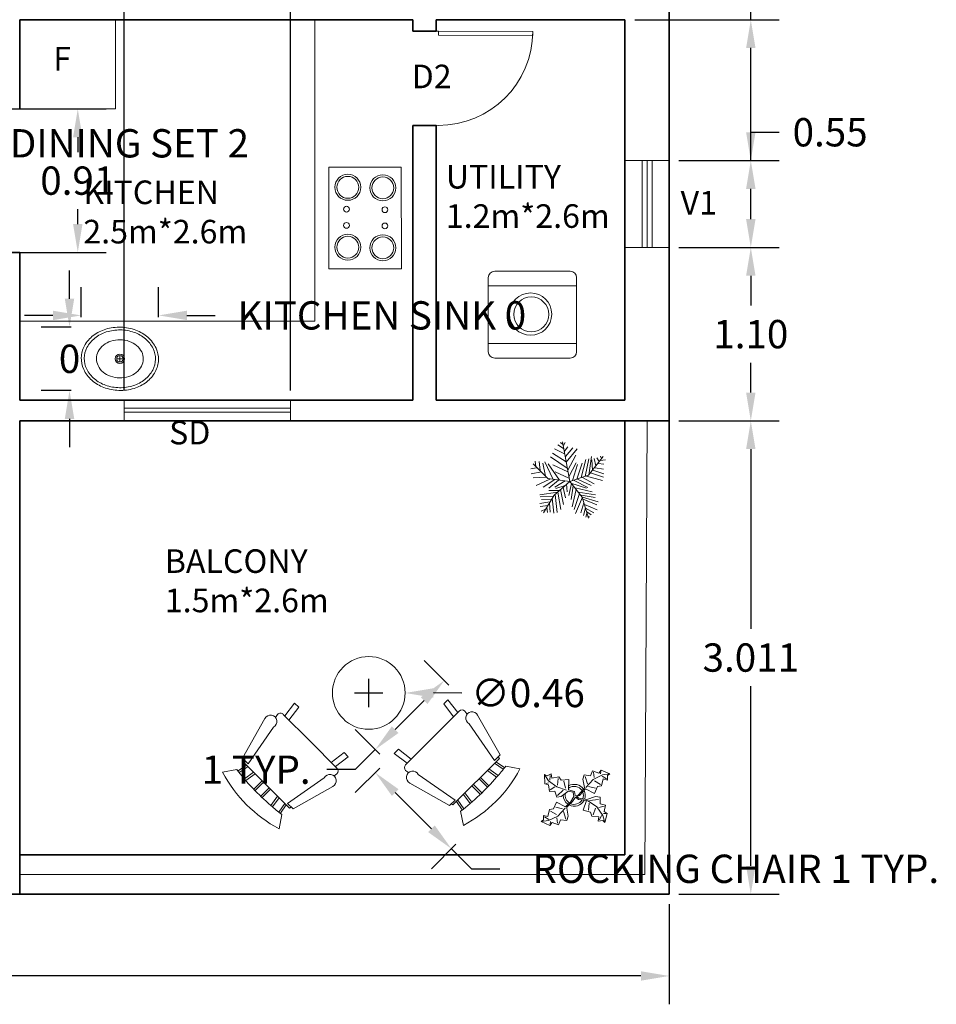
# Model space of a CAD drawing. Units: metres. Extents: x 1988.6 to 2001.1, y 2192 to 2202.5.
# Tile 5 of 6: x 1995.3 to 2001.1, y 2192 to 2198.3. Entities that reach past the tile are written whole.
import ezdxf

# ---------------------------------------------------------------- set-up
doc = ezdxf.new("R2010")
doc.units = ezdxf.units.M
for name, color, linetype, lineweight in [('A-ANNO-DIMS', 2, 'Continuous', 18), ('A-ANNO-TEXT', 7, 'Continuous', 18), ('A-AREA-IDEN', 7, 'Continuous', 18), ('A-DOOR', 3, 'Continuous', 18), ('A-EQPM', 8, 'Continuous', 13), ('A-FLOR-CASE', 9, 'Continuous', 18), ('A-FLOR-FIXT', 9, 'Continuous', 18), ('A-FLOR-HRAL', 4, 'Continuous', 18), ('A-FURN', 9, 'Continuous', 15), ('A-GLAZ', 4, 'Continuous', 18), ('A-PLNT', 94, 'Continuous', 13), ('A-WALL', 7, 'Continuous', 35)]:
    doc.layers.add(name, color=color, linetype=linetype, lineweight=lineweight)
doc.styles.get("Standard").update_dxf_attribs({"font": 'arial.ttf'})
doc.dimstyles.get("Standard").update_dxf_attribs({"dimtxt": 0.18, "dimasz": 0.18, "dimexe": 0.18, "dimexo": 0.0625, "dimgap": 0.09, "dimtad": 0, "dimtih": 1, "dimtoh": 1, "dimdec": 4, "dimzin": 0, "dimdsep": 46, "dimtxsty": 'Standard', "dimcen": 0.09, "dimadec": 0, "dimazin": 0, "dimtfac": 1, "dimtdec": 4, "dimtofl": 0, "dimtmove": 0, "dimatfit": 3, "dimfxl": 1, "dimtolj": 1, "dimtzin": 0, "dimarcsym": 0})

# ---------------------------------------------------------------- blocks, each defined once
blk = doc.blocks.new('Sink - Oval top')
for p, q in [((-1, 0), (1, 0)), ((0, 1), (0, -1))]:
    blk.add_line(p, q)
for points in [[(-12.23, 0.39, 0.117634), (-11.46, -3.36, 0.104469), (-8.88, -6.8, 0.090016), (-5.08, -9.07, 0.08192), (-0.32, -10.02, 0.08192), (4.49, -9.38, 0.090016), (8.42, -7.36, 0.104469), (11.22, -4.09, 0.117634), (12.23, -0.39, 0.117634), (11.46, 3.36, 0.104469), (8.88, 6.8, 0.090016), (5.08, 9.07, 0.08192), (0.32, 10.02, 0.08192), (-4.49, 9.38, 0.090016), (-8.42, 7.36, 0.104469), (-11.22, 4.09, 0.117634)], [(-11.29, 0.16, 0.118622), (-10.52, -3.25, 0.104678), (-8.07, -6.36, 0.089562), (-4.54, -8.37, 0.081185), (-0.13, -9.15, 0.081185), (4.3, -8.49, 0.089562), (7.89, -6.58, 0.104678), (10.42, -3.55, 0.118622), (11.29, -0.16, 0.118622), (10.52, 3.25, 0.104678), (8.07, 6.36, 0.089562), (4.54, 8.37, 0.081185), (0.13, 9.15, 0.081185), (-4.3, 8.49, 0.089562), (-7.89, 6.58, 0.104678), (-10.42, 3.55, 0.118622)], [(-7.42, 0.08, 0.118283), (-6.91, -2.17, 0.104607), (-5.29, -4.21, 0.089718), (-2.97, -5.53, 0.081436), (-0.07, -6.04, 0.081436), (2.84, -5.59, 0.089718), (5.2, -4.33, 0.104607), (6.86, -2.32, 0.118283), (7.42, -0.08, 0.118283), (6.91, 2.17, 0.104607), (5.29, 4.21, 0.089718), (2.97, 5.53, 0.081436), (0.07, 6.04, 0.081436), (-2.84, 5.59, 0.089718), (-5.2, 4.33, 0.104607), (-6.86, 2.32, 0.118283)]]:
    blk.add_lwpolyline(points, format="xyb", close=True)
for radius in [1.5, 1]:
    blk.add_circle((0, 0), radius)
blk = doc.blocks.new('Chair - Rocking')
for p, q in [((-8, -4.5), (-10, -1.5)), ((8, -4.5), (10, -1.5)), ((-7.5, -4.5), (-7, -7)), ((-6.5, -7), (-7.02225, -4.43)), ((-4.5, -7), (-4.96674, -4.19951)), ((-4, -7), (-4.40532, -4.16272)), ((-1.5, -4.05012), (-1.5, -7)), ((-1, -7), (-1, -4.05012)), ((1, -7), (1, -4.04655)), ((1.5, -4.05012), (1.5, -7)), ((4, -7), (4.40187, -4.18694)), ((4.5, -7), (4.96761, -4.19437)), ((6.5, -7), (7, -4.4057)), ((7.5, -4.5), (7, -7)), ((-8.23428, -6.99939), (-8.3093, -7.47958)), ((-8.23041, -7), (8.23915, -7)), ((8.31071, -7.48854), (8.23449, -7.00073)), ((-9, -7.5), (-12, -18.49999)), ((-7, -7.5), (-9, -7.5)), ((-9, -18.49999), (-7, -7.5)), ((7, -7.5), (9, -7.5)), ((9, -18.49999), (7, -7.5)), ((9, -7.5), (12, -18.49999)), ((-10.36644, -20.64523), (-10.5, -21.49999)), ((10.5, -21.49999), (10.3575, -20.58798)), ((-9, -22.49999), (-9.5, -26.49999)), ((0, -22.49999), (-9.5, -22.49999)), ((-8, -26.49999), (-7.5, -22.49999)), ((0, -22.49999), (9.5, -22.49999)), ((8, -26.49999), (7.5, -22.49999)), ((9, -22.49999), (9.5, -26.49999)), ((-9.5, -26.49999), (-8, -26.49999)), ((9.5, -26.49999), (8, -26.49999))]:
    blk.add_line(p, q)
for centre, radius, start, end in [((0, -34.08333), 34.08333, 72.93847, 107.0615), ((0, -68.25004), 64.25, 93.92211, 97.15267), ((0, -68.25004), 64.25, 82.84733, 93.92211), ((-10.5, -18.99999), 1.58114, 161.5651, 18.43495), ((10.5, -18.99999), 1.58114, 161.5651, 18.43495), ((-9.5, -21.49999), 1, 180, 270), ((9.5, -21.49999), 1, 270, 0)]:
    blk.add_arc(centre, radius, start, end)
blk = doc.blocks.new('Plant - Rubber or Philodendron')
for p, q in [((-16.2005, 11.4774), (-13.9899, 8.1064)), ((-16.2005, 11.4774), (-14.8639, 10.7964)), ((-16.0159, 6.3329), (-16.2005, 11.4774)), ((-14.8639, 10.7964), (-12.6195, 11.8975)), ((-13.3174, 8.325), (-13.0735, 11.0065)), ((-12.6195, 11.8975), (-12.1909, 9.4345)), ((4.6914, 8.8812), (5.3859, 11.2828)), ((5.3859, 11.2828), (8.8871, 10.7908)), ((8.8871, 10.7908), (9.9809, 13.4933)), ((9.9809, 13.4933), (13.3837, 12.301)), ((15.3859, 11.3055), (10.3916, 8.7942)), ((10.5828, 12.6946), (10.8893, 9.7953)), ((13.3837, 12.301), (14.68, 13.9039)), ((14.5816, 13.2037), (14.3848, 11.8033)), ((14.68, 13.9039), (19.3848, 11.8146)), ((19.3848, 11.8146), (15.3859, 11.3055)), ((19.3848, 11.8146), (18.1868, 10.9119)), ((18.1868, 10.9119), (18.1925, 8.4119)), ((-14.0069, 5.8704), (-16.0159, 6.3329)), ((-15.3434, 6.5514), (-13.9984, 6.9884)), ((-13.5868, 2.2894), (-14.0069, 5.8704)), ((-13.9899, 8.1064), (-9.5434, 4.7185)), ((-12.1909, 9.4345), (-8.3829, 10.3)), ((-8.8369, 9.409), (-9.0894, 5.6095)), ((-8.3829, 10.3), (-7.0549, 8.501)), ((-7.0549, 8.501), (-3.0284, 8.6941)), ((-4.8529, 4.012), (-5.7184, 7.82)), ((-3.0284, 8.6941), (-3.0709, 3.1041)), ((4.6914, 8.8812), (5.5014, 4.4831)), ((5.9878, 10.4842), (7.1971, 6.3869)), ((10.3916, 8.7942), (6.2847, 4.4028)), ((14.2977, 6.1031), (10.9934, 7.9956)), ((15.7909, 9.1065), (14.8995, 5.3044)), ((15.2875, 10.6053), (17.5907, 9.2105)), ((18.1925, 8.4119), (15.7909, 9.1065)), ((-10.6784, 2.491), (-13.5868, 2.2894)), ((-13.1329, 3.1804), (-10.6614, 4.727)), ((-9.5858, -0.8715), (-10.6784, 2.491)), ((-9.5434, 4.7185), (-4.1917, 2.9888)), ((-9.1318, 0.0195), (-5.9793, 2.9025)), ((-7.1228, -0.443), (-3.5248, 2.2131)), ((-3.5248, 2.2131), (-3.3011, 2.4355)), ((-3.3011, 2.4355), (-0.5306, 1.7947)), ((-3.0709, 3.1041), (0.0797, 2.3163)), ((-0.5306, 1.7947), (-0.2255, -0.5527)), ((-0.5306, 1.7947), (-0.5306, 1.7947)), ((0.0797, 2.3163), (0.4866, -0.031)), ((0.4866, -0.031), (2.1141, 0.2298)), ((2.1141, 0.2298), (5.4346, 3.9146)), ((6.1032, 3.6844), (2.8262, -0.031)), ((5.4346, 3.9146), (5.5014, 4.4831)), ((11.1089, 1.1958), (6.1032, 3.6844)), ((7.7005, 4.8881), (11.5025, 3.9967)), ((12.7005, 4.8994), (11.1089, 1.1958)), ((14.8995, 5.3044), (12.7005, 4.8994)), ((-11.3237, -7.2629), (-9.7321, -3.5593)), ((-9.7321, -3.5593), (-4.7264, -6.0479)), ((-7.1228, -0.443), (-9.5858, -0.8715)), ((-2.019, -3.6148), (-4.7264, -6.0479)), ((-4.0579, -6.2781), (-0.9375, -3.1608)), ((-2.019, -3.6148), (-0.2255, -0.5527)), ((-0.9375, -3.1608), (0.5883, -0.8135)), ((0.5883, -0.8135), (2.2447, -2.0916)), ((2.8262, -0.031), (1.3003, -0.5527)), ((1.3003, -0.5527), (2.4193, -1.4655)), ((2.2447, -2.0916), (6.7108, -2.6626)), ((2.4193, -1.4655), (6.895, -2.1175)), ((4.943, -7.9659), (6.7108, -2.6626)), ((11.6605, -0.5413), (6.895, -2.1175)), ((12.3677, -6.1981), (7.219, -2.6772)), ((8.125, -4.0768), (7.7715, -7.9659)), ((8.3544, -2.7453), (13.1973, -2.1704)), ((11.6605, -0.5413), (14.1354, -0.8948)), ((14.1354, -0.8948), (14.1354, -4.4304)), ((14.1354, -4.4304), (16.9638, -5.1375)), ((16.9638, -5.1375), (16.2567, -8.673)), ((-14.4141, -11.4699), (-13.5228, -7.6679)), ((-13.5228, -7.6679), (-11.3237, -7.2629)), ((-12.921, -8.4665), (-9.6166, -10.359)), ((-6.3237, -7.2516), (-10.1257, -6.3602)), ((-9.0148, -11.1577), (-4.9047, -6.8122)), ((-4.611, -12.8477), (-5.8203, -8.7504)), ((-4.1246, -6.8466), (-4.0579, -6.2781)), ((-3.3146, -11.2447), (-4.1246, -6.8466)), ((8.8321, -9.0266), (4.943, -7.9659)), ((9.5392, -11.1479), (8.8321, -9.0266)), ((10.2463, -10.4408), (11.6605, -6.9053)), ((15.5496, -10.7943), (12.3677, -6.1981)), ((16.2567, -5.8446), (13.4283, -6.5517)), ((17.3174, -9.7337), (15.9032, -9.7337)), ((16.2567, -8.673), (18.0245, -9.7337)), ((18.0245, -9.7337), (16.6103, -14.6834)), ((-18.008, -14.1781), (-16.8101, -13.2754)), ((-18.008, -14.1781), (-14.0091, -13.669)), ((-13.3032, -16.2674), (-18.008, -14.1781)), ((-16.8157, -10.7754), (-14.4141, -11.4699)), ((-16.8101, -13.2754), (-16.8157, -10.7754)), ((-13.9107, -12.9688), (-16.2139, -11.574)), ((-14.0091, -13.669), (-9.0148, -11.1577)), ((-12.0069, -14.6645), (-13.3032, -16.2674)), ((-13.2048, -15.5672), (-13.008, -14.1668)), ((-8.6042, -15.8568), (-12.0069, -14.6645)), ((-9.206, -15.0581), (-9.5126, -12.1588)), ((-7.5103, -13.1543), (-8.6042, -15.8568)), ((-4.0092, -13.6463), (-7.5103, -13.1543)), ((-3.3146, -11.2447), (-4.0092, -13.6463)), ((13.4283, -11.5015), (9.5392, -11.1479)), ((13.0748, -13.9763), (13.4283, -11.5015)), ((15.5496, -13.6228), (13.0748, -13.9763)), ((14.8425, -10.7943), (13.7819, -13.2692)), ((16.6103, -14.6834), (15.5496, -10.7943)), ((16.6103, -14.6834), (15.5496, -13.6228))]:
    blk.add_line(p, q)
for centre, radius, start, end in [((0, 0), 6.1275, 34.37569, 120.1028), ((0.0308, 0.1664), 6, 178.6147, 235.1169), ((0.0308, 0.1664), 5, 168.1647, 238.6725), ((-0.0601, -0.2075), 5.2461, 33.82192, 124.9414), ((-0.2664, 0.1682), 5.2775, 338.4094, 20.03007), ((-0.098, 0.1364), 6.1288, 341.2017, 26.09184), ((-0.0234, 0.3825), 6.1492, 242.5812, 331.2714), ((-0.1102, 0.4886), 5.2883, 247.3711, 327.472)]:
    blk.add_arc(centre, radius, start, end)
blk = doc.blocks.new('*U13')
for p, q in [((0, 0), (0, -6)), ((40, 0), (40, -6))]:
    blk.add_line(p, q)
blk.add_lwpolyline([(0, 0), (0, 40), (1.75, 40), (1.75, 0)], close=True)
blk.add_arc((0, 0), 40, 0, 90)
blk = doc.blocks.new('*U17')
for p, q in [((0, 0), (-266.7, 1447.8)), ((-185.1152, 1008.5578), (-553.1612, 1185.4942)), ((-221.9198, 1197.3052), (-433.5526, 1338.8594)), ((-258.7244, 1362.456), (-332.3336, 1421.4348)), ((-231.1146, 1315.2628), (-166.7002, 1421.4348)), ((-194.31, 1102.9442), (-65.4812, 1256.284)), ((-148.3106, 914.1968), (118.5418, 1220.9018)), ((-129.8956, 701.8528), (265.7602, 1185.4942)), ((-1234.059, 536.7274), (-1252.4486, 737.2604)), ((-1105.2302, 725.4494), (-1077.6458, 395.1732)), ((-93.091, 489.5342), (-700.3796, 902.3858)), ((-129.8956, 713.6638), (-626.7704, 1032.1544)), ((-74.7014, 418.7444), (219.7608, 961.39)), ((412.9786, 147.447), (587.8068, 796.2392)), ((560.197, 182.8292), (698.2206, 819.8358)), ((685.8, 228.6), (1219.2, 914.4)), ((689.0258, 230.0224), (790.2448, 914.1968)), ((808.6344, 784.4282), (827.0494, 418.7444)), ((891.4384, 831.6214), (946.658, 572.1096)), ((983.4626, 867.0036), (1066.2666, 725.4494)), ((1112.2914, 760.8316), (1296.3144, 784.4282)), ((1121.4862, 925.9824), (1149.0706, 831.6214)), ((-1206.4492, 501.3198), (-1418.082, 465.9376)), ((-800.1, 114.3), (-1333.5, 647.7)), ((-976.4268, 666.4706), (-884.4026, 194.6402)), ((-902.8176, 713.6638), (-617.5756, 100.2538)), ((-369.1382, 53.086), (-783.1836, 642.874)), ((-617.5756, 607.4918), (-74.7014, 347.98)), ((-28.6766, 171.0436), (228.9556, 678.2816)), ((100.1268, 41.275), (284.1498, 619.2774)), ((256.5654, 88.4682), (449.7832, 666.4706)), ((845.439, 418.7444), (1241.0948, 277.1902)), ((919.0482, 501.3198), (1222.6798, 454.152)), ((1029.462, 654.685), (1241.0948, 631.0884)), ((-1031.621, 347.98), (-1399.667, 277.1902)), ((-847.598, 159.2326), (-1326.0578, 135.636)), ((-718.7946, 88.4682), (-1215.644, -147.447)), ((-543.9664, 76.6572), (-967.2066, -206.4512)), ((0, 0), (-800.1, 114.3)), ((-405.9428, 53.086), (-764.794, -241.8334)), ((0, 0), (-571.5, -495.3)), ((-166.7002, 29.4894), (-543.9664, -206.4512)), ((-525.5514, 347.98), (-28.6766, 123.8504)), ((0, 0), (685.8, 228.6)), ((0, 0), (457.2, -571.5)), ((164.5412, 41.275), (661.416, -218.2368)), ((284.1498, 88.4682), (781.0246, -147.447)), ((458.978, 147.447), (891.4384, -88.4682)), ((615.4166, 194.6402), (1185.8752, 41.275)), ((753.4148, 312.5978), (1222.6798, 159.2326)), ((-387.5278, -324.4088), (-764.794, -324.4088)), ((-166.7002, -147.447), (-507.1618, -253.619)), ((-341.5284, -289.0012), (-221.9198, -831.6214)), ((-240.3094, -218.2368), (-157.5054, -595.7062)), ((-120.7008, -88.4682), (-93.091, -371.5766)), ((63.3222, -76.6826), (-37.8714, -513.1308)), ((44.9326, -64.897), (615.4166, -241.8334)), ((127.7366, -159.258), (54.1274, -654.685)), ((228.9556, -289.0012), (90.932, -914.1968)), ((192.151, -230.0224), (817.8292, -371.5766)), ((-442.7474, -383.3876), (-1086.8406, -477.7486)), ((-617.5756, -548.5384), (-1077.6458, -560.324)), ((-681.9646, -666.496), (-1022.4262, -654.685)), ((-571.5, -495.3), (-952.5, -1143)), ((-635.9652, -607.5172), (-580.771, -1150.1374)), ((-525.5514, -465.963), (-451.9422, -1126.5408)), ((-433.5526, -383.3876), (-323.1134, -1020.3688)), ((357.759, -430.5554), (164.5412, -1020.3688)), ((458.978, -572.1096), (210.5406, -1161.923)), ((311.7596, -383.3876), (937.4378, -477.7486)), ((412.9786, -501.3452), (919.0482, -583.9206)), ((457.2, -571.5), (685.8, -1333.5)), ((468.1982, -572.1096), (1029.462, -737.2604)), ((486.5878, -642.8994), (983.4626, -843.4324)), ((-718.7946, -737.2604), (-1086.8406, -796.2392)), ((-783.1836, -867.029), (-1077.6458, -902.4112)), ((-875.2078, -1008.5832), (-1040.8412, -1079.3476)), ((-829.2084, -937.7934), (-810.7934, -1126.5408)), ((-737.1842, -784.4536), (-709.5744, -1114.7298)), ((514.1976, -772.6426), (403.7838, -1138.3264)), ((578.612, -961.39), (495.7826, -1232.7128)), ((541.8074, -831.6214), (992.6574, -1032.1544)), ((578.612, -973.1756), (873.0488, -1138.3264)), ((624.6114, -1161.923), (587.8068, -1291.6916)), ((624.6114, -1102.9442), (781.0246, -1209.1162)), ((679.8056, -1268.095), (716.6102, -1291.6916))]:
    blk.add_line(p, q)
blk = doc.blocks.new('*D30')
at = {"layer": 'A-ANNO-DIMS', "color": 0, "lineweight": -2, "transparency": 16777216}
for p, q in [((1997.5406, 2193.5067), (1997.3848, 2193.3508)), ((1997.6393, 2193.3508), (1997.8697, 2193.1205)), ((1998.0255, 2193.0217), (1997.8697, 2192.8659)), ((1997.997, 2192.9932), (1998.1243, 2192.8659)), ((1998.1243, 2192.8659), (1998.3043, 2192.8659))]:
    blk.add_line(p, q, dxfattribs=at)
at = {"layer": 'A-ANNO-DIMS', "color": 0, "transparency": 16777216}
for points in [[(1997.6605, 2193.3721), (1997.6181, 2193.3296), (1997.512, 2193.4781)], [(1997.8909, 2193.1417), (1997.8485, 2193.0993), (1997.997, 2192.9932)]]:
    blk.add_solid(points, dxfattribs=at)
at = {"layer": 'Defpoints', "color": 0, "transparency": 16777216}
for p in [(1997.5848, 2193.5509), (1998.0697, 2193.0659), (1997.997, 2192.9932)]:
    blk.add_point(p, dxfattribs=at)
at = {"layer": 'A-ANNO-DIMS', "color": 0, "transparency": 16777216, "insert": (1999.8056, 2192.8659), "char_height": 0.18, "attachment_point": 5}
blk.add_mtext('\\A1;ROCKING CHAIR 1 TYP.', dxfattribs=at)
blk = doc.blocks.new('*D31')
at = {"layer": 'A-ANNO-DIMS', "color": 0, "lineweight": -2, "transparency": 16777216}
for p, q in [((1997.9795, 2194.0339), (1997.8236, 2194.1898)), ((1997.8236, 2193.9352), (1997.6393, 2193.7509)), ((1997.5406, 2193.5951), (1997.3848, 2193.7509)), ((1997.512, 2193.6236), (1997.3848, 2193.4963)), ((1997.3848, 2193.4963), (1997.2048, 2193.4963))]:
    blk.add_line(p, q, dxfattribs=at)
at = {"layer": 'A-ANNO-DIMS', "color": 0, "transparency": 16777216}
for points in [[(1997.8024, 2193.9564), (1997.8448, 2193.914), (1997.9509, 2194.0625)], [(1997.6181, 2193.7721), (1997.6605, 2193.7297), (1997.512, 2193.6236)]]:
    blk.add_solid(points, dxfattribs=at)
at = {"layer": 'Defpoints', "color": 0, "transparency": 16777216}
for p in [(1998.0237, 2193.9897), (1997.512, 2193.6236), (1997.5848, 2193.5509)]:
    blk.add_point(p, dxfattribs=at)
at = {"layer": 'A-ANNO-DIMS', "color": 0, "transparency": 16777216, "insert": (1996.7551, 2193.4963), "char_height": 0.18, "attachment_point": 5}
blk.add_mtext('\\A1;1 TYP.', dxfattribs=at)
blk = doc.blocks.new('*D44')
at = {"layer": 'A-ANNO-DIMS', "color": 0, "lineweight": -2, "transparency": 16777216}
for p, q in [((1995.6416, 2196.3734), (1995.6416, 2196.5648)), ((1996.1345, 2196.3734), (1996.1345, 2196.5648)), ((1995.4616, 2196.3848), (1995.2816, 2196.3848)), ((1996.3145, 2196.3848), (1996.4945, 2196.3848))]:
    blk.add_line(p, q, dxfattribs=at)
at = {"layer": 'A-ANNO-DIMS', "color": 0, "transparency": 16777216}
for points in [[(1995.4616, 2196.4148), (1995.4616, 2196.3548), (1995.6416, 2196.3848)], [(1996.3145, 2196.4148), (1996.3145, 2196.3548), (1996.1345, 2196.3848)]]:
    blk.add_solid(points, dxfattribs=at)
at = {"layer": 'Defpoints', "color": 0, "transparency": 16777216}
for p in [(1996.1345, 2196.3848), (1995.6416, 2196.3109), (1996.1345, 2196.3109)]:
    blk.add_point(p, dxfattribs=at)
at = {"layer": 'A-ANNO-DIMS', "color": 0, "transparency": 16777216, "insert": (1997.5543, 2196.3848), "char_height": 0.18, "attachment_point": 5}
blk.add_mtext('\\A1;KITCHEN SINK 0', dxfattribs=at)
blk = doc.blocks.new('*D45')
at = {"layer": 'A-ANNO-DIMS', "color": 0, "lineweight": -2, "transparency": 16777216}
for p, q in [((1995.5677, 2196.4909), (1995.5677, 2196.6709)), ((1995.5791, 2196.3109), (1995.3877, 2196.3109)), ((1995.5791, 2195.9066), (1995.3877, 2195.9066)), ((1995.5677, 2195.7266), (1995.5677, 2195.5466))]:
    blk.add_line(p, q, dxfattribs=at)
at = {"layer": 'A-ANNO-DIMS', "color": 0, "transparency": 16777216}
for points in [[(1995.5377, 2196.4909), (1995.5977, 2196.4909), (1995.5677, 2196.3109)], [(1995.5377, 2195.7266), (1995.5977, 2195.7266), (1995.5677, 2195.9066)]]:
    blk.add_solid(points, dxfattribs=at)
at = {"layer": 'Defpoints', "color": 0, "transparency": 16777216}
for p in [(1995.5677, 2196.3109), (1995.6416, 2196.3109), (1995.6416, 2195.9066)]:
    blk.add_point(p, dxfattribs=at)
at = {"layer": 'A-ANNO-DIMS', "color": 0, "transparency": 16777216, "insert": (1995.5677, 2196.1088), "char_height": 0.18, "attachment_point": 5}
blk.add_mtext('\\A1;0', dxfattribs=at)
blk = doc.blocks.new('*D46')
at = {"layer": 'A-ANNO-DIMS', "color": 0, "lineweight": -2, "transparency": 16777216}
for p, q in [((1993.2119, 2197.2927), (1993.2119, 2197.659)), ((1994.8706, 2197.2927), (1994.8706, 2197.659)), ((1993.3919, 2197.479), (1994.6906, 2197.479)), ((1994.8706, 2197.479), (1995.0506, 2197.479))]:
    blk.add_line(p, q, dxfattribs=at)
at = {"layer": 'A-ANNO-DIMS', "color": 0, "transparency": 16777216}
for points in [[(1993.3919, 2197.509), (1993.3919, 2197.449), (1993.2119, 2197.479)], [(1994.6906, 2197.509), (1994.6906, 2197.449), (1994.8706, 2197.479)]]:
    blk.add_solid(points, dxfattribs=at)
at = {"layer": 'Defpoints', "color": 0, "transparency": 16777216}
for p in [(1994.8706, 2197.479), (1993.2119, 2197.2302), (1994.8706, 2197.2302)]:
    blk.add_point(p, dxfattribs=at)
at = {"layer": 'A-ANNO-DIMS', "color": 0, "transparency": 16777216, "insert": (1995.9486, 2197.479), "char_height": 0.18, "attachment_point": 5}
blk.add_mtext('\\A1;DINING SET 2', dxfattribs=at)
blk = doc.blocks.new('*D52')
at = {"layer": 'A-ANNO-DIMS', "color": 0, "lineweight": -2, "transparency": 16777216}
for p, q in [((1989.3818, 2192.6413), (1989.3818, 2192.0043)), ((1999.3818, 2192.6413), (1999.3818, 2192.0043)), ((1989.5618, 2192.1843), (1994.1717, 2192.1843)), ((1999.2018, 2192.1843), (1994.592, 2192.1843))]:
    blk.add_line(p, q, dxfattribs=at)
at = {"layer": 'A-ANNO-DIMS', "color": 0, "transparency": 16777216}
for points in [[(1989.5618, 2192.2143), (1989.5618, 2192.1543), (1989.3818, 2192.1843)], [(1999.2018, 2192.2143), (1999.2018, 2192.1543), (1999.3818, 2192.1843)]]:
    blk.add_solid(points, dxfattribs=at)
at = {"layer": 'Defpoints', "color": 0, "transparency": 16777216}
for p in [(1989.3818, 2192.7038), (1999.3818, 2192.7038), (1999.3818, 2192.1843)]:
    blk.add_point(p, dxfattribs=at)
at = {"layer": 'A-ANNO-DIMS', "color": 0, "transparency": 16777216, "insert": (1994.3818, 2192.1843), "char_height": 0.18, "attachment_point": 5}
blk.add_mtext('\\A1;10', dxfattribs=at)
blk = doc.blocks.new('*D68')
at = {"layer": 'A-ANNO-DIMS', "color": 0, "lineweight": -2, "transparency": 16777216}
for p, q in [((1999.4443, 2195.7145), (2000.0813, 2195.7145)), ((1999.9013, 2195.5345), (1999.9013, 2194.3911)), ((1999.9013, 2192.8838), (1999.9013, 2194.0272)), ((1999.4443, 2192.7038), (2000.0813, 2192.7038))]:
    blk.add_line(p, q, dxfattribs=at)
at = {"layer": 'A-ANNO-DIMS', "color": 0, "transparency": 16777216}
for points in [[(1999.8713, 2195.5345), (1999.9313, 2195.5345), (1999.9013, 2195.7145)], [(1999.8713, 2192.8838), (1999.9313, 2192.8838), (1999.9013, 2192.7038)]]:
    blk.add_solid(points, dxfattribs=at)
at = {"layer": 'Defpoints', "color": 0, "transparency": 16777216}
for p in [(1999.3818, 2195.7145), (1999.9013, 2195.7145), (1999.3818, 2192.7038)]:
    blk.add_point(p, dxfattribs=at)
at = {"layer": 'A-ANNO-DIMS', "color": 0, "transparency": 16777216, "insert": (1999.9013, 2194.2091), "char_height": 0.18, "attachment_point": 5}
blk.add_mtext('\\A1;3.011', dxfattribs=at)
blk = doc.blocks.new('*D69')
at = {"layer": 'A-ANNO-DIMS', "color": 0, "lineweight": -2, "transparency": 16777216}
for p, q in [((1999.4443, 2196.817), (2000.0813, 2196.817)), ((1999.9013, 2196.637), (1999.9013, 2196.4476)), ((1999.9013, 2195.8945), (1999.9013, 2196.0838)), ((1999.4443, 2195.7145), (2000.0813, 2195.7145))]:
    blk.add_line(p, q, dxfattribs=at)
at = {"layer": 'A-ANNO-DIMS', "color": 0, "transparency": 16777216}
for points in [[(1999.8713, 2196.637), (1999.9313, 2196.637), (1999.9013, 2196.817)], [(1999.8713, 2195.8945), (1999.9313, 2195.8945), (1999.9013, 2195.7145)]]:
    blk.add_solid(points, dxfattribs=at)
at = {"layer": 'Defpoints', "color": 0, "transparency": 16777216}
for p in [(1999.3818, 2196.817), (1999.9013, 2196.817), (1999.3818, 2195.7145)]:
    blk.add_point(p, dxfattribs=at)
at = {"layer": 'A-ANNO-DIMS', "color": 0, "transparency": 16777216, "insert": (1999.9013, 2196.2657), "char_height": 0.18, "attachment_point": 5}
blk.add_mtext('\\A1;1.10', dxfattribs=at)
blk = doc.blocks.new('*D70')
at = {"layer": 'A-ANNO-DIMS', "color": 0, "lineweight": -2, "transparency": 16777216}
for p, q in [((1999.9013, 2197.3693), (1999.9013, 2197.5493)), ((1999.9013, 2197.5493), (2000.0813, 2197.5493)), ((1999.4443, 2197.3693), (2000.0813, 2197.3693)), ((1999.9013, 2196.997), (1999.9013, 2197.1893)), ((1999.4443, 2196.817), (2000.0813, 2196.817))]:
    blk.add_line(p, q, dxfattribs=at)
at = {"layer": 'A-ANNO-DIMS', "color": 0, "transparency": 16777216}
for points in [[(1999.8713, 2197.1893), (1999.9313, 2197.1893), (1999.9013, 2197.3693)], [(1999.8713, 2196.997), (1999.9313, 2196.997), (1999.9013, 2196.817)]]:
    blk.add_solid(points, dxfattribs=at)
at = {"layer": 'Defpoints', "color": 0, "transparency": 16777216}
for p in [(1999.3818, 2197.3693), (1999.9013, 2197.3693), (1999.3818, 2196.817)]:
    blk.add_point(p, dxfattribs=at)
at = {"layer": 'A-ANNO-DIMS', "color": 0, "transparency": 16777216, "insert": (2000.4058, 2197.5493), "char_height": 0.18, "attachment_point": 5}
blk.add_mtext('\\A1;0.55', dxfattribs=at)
blk = doc.blocks.new('*D71')
at = {"layer": 'A-ANNO-DIMS', "color": 0, "lineweight": -2, "transparency": 16777216}
for p, q in [((1999.9013, 2198.2651), (1999.9013, 2198.4451)), ((1999.9013, 2198.4451), (2000.0813, 2198.4451)), ((1999.1632, 2198.2651), (2000.0813, 2198.2651)), ((1999.9013, 2197.5493), (1999.9013, 2198.0851)), ((1999.4443, 2197.3693), (2000.0813, 2197.3693))]:
    blk.add_line(p, q, dxfattribs=at)
at = {"layer": 'A-ANNO-DIMS', "color": 0, "transparency": 16777216}
for points in [[(1999.8713, 2198.0851), (1999.9313, 2198.0851), (1999.9013, 2198.2651)], [(1999.8713, 2197.5493), (1999.9313, 2197.5493), (1999.9013, 2197.3693)]]:
    blk.add_solid(points, dxfattribs=at)
at = {"layer": 'Defpoints', "color": 0, "transparency": 16777216}
for p in [(1999.1007, 2198.2651), (1999.9013, 2198.2651), (1999.3818, 2197.3693)]:
    blk.add_point(p, dxfattribs=at)
at = {"layer": 'A-ANNO-DIMS', "color": 0, "transparency": 16777216, "insert": (2000.4048, 2198.4451), "char_height": 0.18, "attachment_point": 5}
blk.add_mtext('\\A1;0.90', dxfattribs=at)
blk = doc.blocks.new('*D74')
at = {"layer": 'A-ANNO-DIMS', "color": 0, "lineweight": -2, "transparency": 16777216}
for p, q in [((1995.9155, 2195.9076), (1995.9155, 2202.4533)), ((1996.9733, 2195.9076), (1996.9733, 2202.4533)), ((1995.7355, 2202.2733), (1995.5555, 2202.2733)), ((1997.1533, 2202.2733), (1997.3333, 2202.2733))]:
    blk.add_line(p, q, dxfattribs=at)
at = {"layer": 'A-ANNO-DIMS', "color": 0, "transparency": 16777216}
for points in [[(1995.7355, 2202.3033), (1995.7355, 2202.2433), (1995.9155, 2202.2733)], [(1997.1533, 2202.3033), (1997.1533, 2202.2433), (1996.9733, 2202.2733)]]:
    blk.add_solid(points, dxfattribs=at)
at = {"layer": 'Defpoints', "color": 0, "transparency": 16777216}
for p in [(1996.9733, 2202.2733), (1995.9155, 2195.8451), (1996.9733, 2195.8451)]:
    blk.add_point(p, dxfattribs=at)
at = {"layer": 'A-ANNO-DIMS', "color": 0, "transparency": 16777216, "insert": (1996.4444, 2202.2733), "char_height": 0.18, "attachment_point": 5}
blk.add_mtext('\\A1;1.06', dxfattribs=at)
blk = doc.blocks.new('*D77')
at = {"layer": 'A-ANNO-DIMS', "color": 0, "lineweight": -2, "transparency": 16777216}
for p, q in [((1995.1632, 2197.698), (1995.8002, 2197.698)), ((1995.6202, 2197.518), (1995.6202, 2197.4236)), ((1995.6202, 2196.9654), (1995.6202, 2197.0598)), ((1995.1632, 2196.7854), (1995.8002, 2196.7854))]:
    blk.add_line(p, q, dxfattribs=at)
at = {"layer": 'A-ANNO-DIMS', "color": 0, "transparency": 16777216}
for points in [[(1995.5902, 2197.518), (1995.6502, 2197.518), (1995.6202, 2197.698)], [(1995.5902, 2196.9654), (1995.6502, 2196.9654), (1995.6202, 2196.7854)]]:
    blk.add_solid(points, dxfattribs=at)
at = {"layer": 'Defpoints', "color": 0, "transparency": 16777216}
for p in [(1995.1007, 2197.698), (1995.1007, 2196.7854), (1995.6202, 2196.7854)]:
    blk.add_point(p, dxfattribs=at)
at = {"layer": 'A-ANNO-DIMS', "color": 0, "transparency": 16777216, "insert": (1995.6202, 2197.2417), "char_height": 0.18, "attachment_point": 5}
blk.add_mtext('\\A1;0.91', dxfattribs=at)
blk = doc.blocks.new('*D80')
at = {"layer": 'A-ANNO-DIMS', "color": 0, "lineweight": -2, "transparency": 16777216}
for p, q in [((1997.4712, 2193.8942), (1997.4712, 2194.0742)), ((1997.3812, 2193.9842), (1997.5612, 2193.9842)), ((1998.0626, 2193.9837), (1997.8826, 2193.9839))]:
    blk.add_line(p, q, dxfattribs=at)
at = {"layer": 'A-ANNO-DIMS', "color": 0, "transparency": 16777216}
blk.add_solid([(1997.8826, 2194.0139), (1997.8826, 2193.9539), (1997.7026, 2193.984)], dxfattribs=at)
at = {"layer": 'Defpoints', "color": 0, "transparency": 16777216}
for p in [(1997.2397, 2193.9843), (1997.7026, 2193.984)]:
    blk.add_point(p, dxfattribs=at)
at = {"layer": 'A-ANNO-DIMS', "color": 0, "transparency": 16777216, "insert": (1998.4842, 2193.9837), "char_height": 0.18, "attachment_point": 5}
blk.add_mtext('\\A1;∅0.46', dxfattribs=at)

msp = doc.modelspace()

# ---------------------------------------------------------------- linework, layer by layer
at = {"layer": 'A-DOOR'}
for p, q in [((1995.9155, 2195.8451), (1996.9733, 2195.8451)), ((1995.9155, 2195.8451), (1995.9155, 2195.7145)), ((1995.9155, 2195.7947), (1996.9733, 2195.7947)), ((1996.9733, 2195.8451), (1996.9733, 2195.7145)), ((1996.9733, 2195.7695), (1995.9155, 2195.7695))]:
    msp.add_line(p, q, dxfattribs=at)
at = {"layer": 'A-EQPM'}
for p, q in [((1995.86, 2198.2651), (1995.86, 2197.698)), ((1995.86, 2197.698), (1995.1007, 2197.698)), ((1998.2722, 2196.6658), (1998.7524, 2196.6658)), ((1998.2314, 2196.154), (1998.2314, 2196.625)), ((1998.7932, 2196.625), (1998.7932, 2196.154)), ((1998.2314, 2196.5722), (1998.7932, 2196.5722)), ((1998.2314, 2196.2067), (1998.7932, 2196.2067)), ((1998.7524, 2196.1131), (1998.2722, 2196.1131))]:
    msp.add_line(p, q, dxfattribs=at)
msp.add_lwpolyline([(1997.2164, 2197.3277), (1997.6764, 2197.3277), (1997.6786, 2196.6814), (1997.2164, 2196.6814)], close=True, dxfattribs=at)
for centre, radius in [((1997.338, 2197.1994), 0.0826), ((1997.338, 2197.1994), 0.0696), ((1997.5607, 2197.1958), 0.0826), ((1997.5607, 2197.1958), 0.0696), ((1997.3295, 2197.0605), 0.0184), ((1997.574, 2197.057), 0.0184), ((1997.3295, 2196.9572), 0.0184), ((1997.574, 2196.9536), 0.0184), ((1997.338, 2196.8183), 0.0826), ((1997.338, 2196.8183), 0.0696), ((1997.5607, 2196.8148), 0.0826), ((1997.5607, 2196.8148), 0.0696), ((1998.5006, 2196.3927), 0.1345), ((1998.5049, 2196.3912), 0.111)]:
    msp.add_circle(centre, radius, dxfattribs=at)
for centre, start, end in [((1998.2722, 2196.625), 90, 180), ((1998.7524, 2196.625), 0, 90), ((1998.2722, 2196.154), 180, 270), ((1998.7524, 2196.154), 270, 0)]:
    msp.add_arc(centre, 0.0408, start, end, dxfattribs=at)
at = {"layer": 'A-FLOR-CASE'}
for p, q in [((1997.1281, 2198.2651), (1997.1281, 2196.3471)), ((1997.1281, 2196.3471), (1995.2507, 2196.3471))]:
    msp.add_line(p, q, dxfattribs=at)
at = {"layer": 'A-FLOR-HRAL'}
for p, q in [((1999.2262, 2192.8288), (1999.2412, 2195.7145)), ((1995.2507, 2192.8288), (1999.2262, 2192.8288))]:
    msp.add_line(p, q, dxfattribs=at)
at = {"layer": 'A-FURN'}
msp.add_circle((1997.4712, 2193.9842), 0.2314, dxfattribs=at)
at = {"layer": 'A-GLAZ'}
for p, q in [((1999.1007, 2197.3693), (1999.3818, 2197.3693)), ((1999.2101, 2197.3693), (1999.2101, 2196.817)), ((1999.2412, 2197.3693), (1999.2412, 2196.817)), ((1999.2735, 2197.3693), (1999.2735, 2196.817)), ((1999.1007, 2196.817), (1999.3818, 2196.817))]:
    msp.add_line(p, q, dxfattribs=at)
at = {"layer": 'A-WALL'}
for p, q in [((1999.3818, 2192.7038), (1999.3818, 2201.7538)), ((1997.7507, 2198.2651), (1995.2507, 2198.2651)), ((1995.2507, 2197.698), (1995.2507, 2198.2651)), ((1997.7507, 2198.1924), (1997.7507, 2198.2651)), ((1999.1007, 2198.2651), (1997.9007, 2198.2651)), ((1997.9007, 2198.1924), (1997.9007, 2198.2651)), ((1999.1007, 2195.8451), (1999.1007, 2198.2651)), ((1997.7507, 2198.1924), (1997.9007, 2198.1924)), ((1997.9007, 2197.5933), (1997.7507, 2197.5933)), ((1997.7507, 2197.5933), (1997.7507, 2197.5836)), ((1997.7507, 2195.8451), (1997.7507, 2197.5836)), ((1997.9007, 2195.8451), (1997.9007, 2197.5933)), ((1995.1007, 2196.7854), (1995.2507, 2196.7854)), ((1995.2507, 2195.8451), (1995.2507, 2196.7854)), ((1997.7507, 2195.8451), (1995.2507, 2195.8451)), ((1999.1007, 2195.8451), (1997.9007, 2195.8451)), ((1999.1007, 2195.7145), (1995.2507, 2195.7145)), ((1995.2507, 2192.9538), (1995.2507, 2195.7145)), ((1999.1007, 2192.9538), (1999.1007, 2195.7145)), ((1999.1007, 2195.7145), (1999.3818, 2195.7145)), ((1995.2507, 2192.9538), (1999.1007, 2192.9538)), ((1995.2507, 2192.9538), (1995.2507, 2192.7038)), ((1990.7282, 2192.7038), (1999.3818, 2192.7038))]:
    msp.add_line(p, q, dxfattribs=at)

# ---------------------------------------------------------------- block references
at = {"layer": 'A-DOOR', "xscale": 0.0149691911654328, "yscale": 0.0149691911654328, "zscale": 0.0149691911654328, "rotation": 269.7935336429091}
msp.add_blockref('*U13', (1997.9155, 2198.192), dxfattribs=at)
at = {"layer": 'A-FLOR-FIXT', "xscale": 0.0200750651153481, "yscale": 0.0200750651153481, "zscale": 0.0200750651153481}
msp.add_blockref('Sink - Oval top', (1995.888, 2196.1088), dxfattribs=at)
at = {"layer": 'A-FURN', "xscale": 0.0254, "yscale": 0.0254, "zscale": 0.0254}
for p, rotation in [((1998.2802, 2193.2943), 225.0000000000197), ((1996.6941, 2193.2731), 134.9999999999782)]:
    msp.add_blockref('Chair - Rocking', p, dxfattribs=dict(at, rotation=rotation))
at = {"layer": 'A-PLNT'}
for name, p, xscale, yscale, zscale in [('*U17', (1998.7495, 2195.3284), 0.0001749914222183, 0.0001749914222183, 0.0001749914222183), ('Plant - Rubber or Philodendron', (1998.7783, 2193.3314), 0.0116630215705542, 0.0116630215705542, 0.0116630215705542)]:
    msp.add_blockref(name, p, dxfattribs=dict(at, xscale=xscale, yscale=yscale, zscale=zscale))

# ---------------------------------------------------------------- texts
at = {"layer": 'A-ANNO-TEXT', "char_height": 0.15, "attachment_point": 1}
for s, insert in [('F', (1995.4644, 2198.0919)), ('D2', (1997.7438, 2197.9791)), ('V1', (1999.4547, 2197.1763)), ('SD', (1996.2012, 2195.7145))]:
    msp.add_mtext_dynamic_manual_height_columns(s, width=0.386628, gutter_width=12.5, heights=[0], dxfattribs=dict(at, insert=insert))
at = {"layer": 'A-AREA-IDEN', "char_height": 0.15, "attachment_point": 1}
for s, insert in [('UTILITY\\P1.2m*2.6m', (1997.9613, 2197.3415)), ('KITCHEN\\P2.5m*2.6m', (1995.6555, 2197.2424)), ('BALCONY\\P1.5m*2.6m', (1996.1738, 2194.8974))]:
    msp.add_mtext_dynamic_manual_height_columns(s, width=0.386628, gutter_width=12.5, heights=[0], dxfattribs=dict(at, insert=insert))

# ---------------------------------------------------------------- dimensions: what is measured, and where the dimension line sits
at = {"layer": 'A-ANNO-DIMS'}
for base, p1, p2, override, picture, middle in [((1996.9733, 2202.2733), (1995.9155, 2195.8451), (1996.9733, 2195.8451), {"dimdec": 2, "dimlfac": 1, "dimrnd": 0, "dimzin": 0, "dimdsep": 46, "dimlunit": 2}, '*D74', (1996.4444, 2202.2733)), ((1999.3818, 2192.1843), (1989.3818, 2192.7038), (1999.3818, 2192.7038), {"dimdec": 0, "dimlfac": 1, "dimrnd": 0, "dimzin": 0, "dimdsep": 46, "dimlunit": 2}, '*D52', (1994.3818, 2192.1843))]:
    dim = msp.add_linear_dim(base=base, p1=p1, p2=p2, dimstyle='Standard', override=override, dxfattribs=at)
    dim.commit()
    dim.dimension.update_dxf_attribs({"geometry": picture, "text_midpoint": middle})
for base, p1, p2, angle, override, picture, middle in [((1999.9013, 2198.2651), (1999.3818, 2197.3693), (1999.1007, 2198.2651), 90, {"dimdec": 2, "dimlfac": 1, "dimrnd": 0, "dimzin": 0, "dimdsep": 46, "dimlunit": 2}, '*D71', (2000.4048, 2198.4451)), ((1995.6202, 2196.7854), (1995.1007, 2197.698), (1995.1007, 2196.7854), 270, {"dimdec": 2, "dimlfac": 1, "dimrnd": 0, "dimzin": 0, "dimdsep": 46, "dimlunit": 2}, '*D77', (1995.6202, 2197.2417)), ((1999.9013, 2197.3693), (1999.3818, 2196.817), (1999.3818, 2197.3693), 90, {"dimdec": 2, "dimlfac": 1, "dimrnd": 0, "dimzin": 0, "dimdsep": 46, "dimlunit": 2}, '*D70', (2000.4058, 2197.5493)), ((1999.9013, 2196.817), (1999.3818, 2195.7145), (1999.3818, 2196.817), 90, {"dimdec": 2, "dimlfac": 1, "dimrnd": 0, "dimzin": 0, "dimdsep": 46, "dimlunit": 2}, '*D69', (1999.9013, 2196.2657)), ((1995.5677, 2196.3109), (1995.6416, 2195.9066), (1995.6416, 2196.3109), 90, {"dimdec": 0, "dimlfac": 1, "dimrnd": 0, "dimzin": 0, "dimdsep": 46, "dimlunit": 2}, '*D45', (1995.5677, 2196.1088)), ((1999.9013, 2195.7145), (1999.3818, 2192.7038), (1999.3818, 2195.7145), 90, {"dimdec": 3, "dimlfac": 1, "dimrnd": 0, "dimzin": 0, "dimdsep": 46, "dimlunit": 2}, '*D68', (1999.9013, 2194.2091))]:
    dim = msp.add_linear_dim(base=base, p1=p1, p2=p2, angle=angle, dimstyle='Standard', override=override, dxfattribs=at)
    dim.commit()
    dim.dimension.update_dxf_attribs({"geometry": picture, "text_midpoint": middle})
for base, p1, p2, text, picture, middle in [((1994.8706, 2197.479), (1993.2119, 2197.2302), (1994.8706, 2197.2302), 'DINING SET <>', '*D46', (1995.9486, 2197.479)), ((1996.1345, 2196.3848), (1995.6416, 2196.3109), (1996.1345, 2196.3109), 'KITCHEN SINK <>', '*D44', (1997.5543, 2196.3848))]:
    dim = msp.add_linear_dim(base=base, p1=p1, p2=p2, text=text, dimstyle='Standard', override={"dimdec": 0, "dimlfac": 1, "dimrnd": 0, "dimzin": 0, "dimdsep": 46, "dimlunit": 2}, dxfattribs=at)
    dim.commit()
    dim.dimension.update_dxf_attribs({"geometry": picture, "text_midpoint": middle})
for base, p1, p2, angle, text, picture, middle in [((1997.512, 2193.6236), (1998.0237, 2193.9897), (1997.5848, 2193.5509), 225, '<> TYP.', '*D31', (1996.7551, 2193.4963)), ((1997.997, 2192.9932), (1997.5848, 2193.5509), (1998.0697, 2193.0659), 315, 'ROCKING CHAIR <> TYP.', '*D30', (1999.8056, 2192.8659))]:
    dim = msp.add_linear_dim(base=base, p1=p1, p2=p2, angle=angle, text=text, dimstyle='Standard', override={"dimdec": 0, "dimlfac": 1, "dimrnd": 0, "dimzin": 0, "dimdsep": 46, "dimlunit": 2}, dxfattribs=at)
    dim.commit()
    dim.dimension.update_dxf_attribs({"geometry": picture, "text_midpoint": middle})
dim = msp.add_diameter_dim_2p(p1=(1997.2397, 2193.9843), p2=(1997.7026, 2193.984), dimstyle='Standard', override={"dimdec": 2, "dimlfac": 1, "dimrnd": 0, "dimzin": 0, "dimdsep": 46, "dimlunit": 2}, dxfattribs=at)
dim.commit()
dim.dimension.update_dxf_attribs({"geometry": '*D80', "text_midpoint": (1998.0626, 2193.9837)})

doc.saveas('drawing.dxf')
